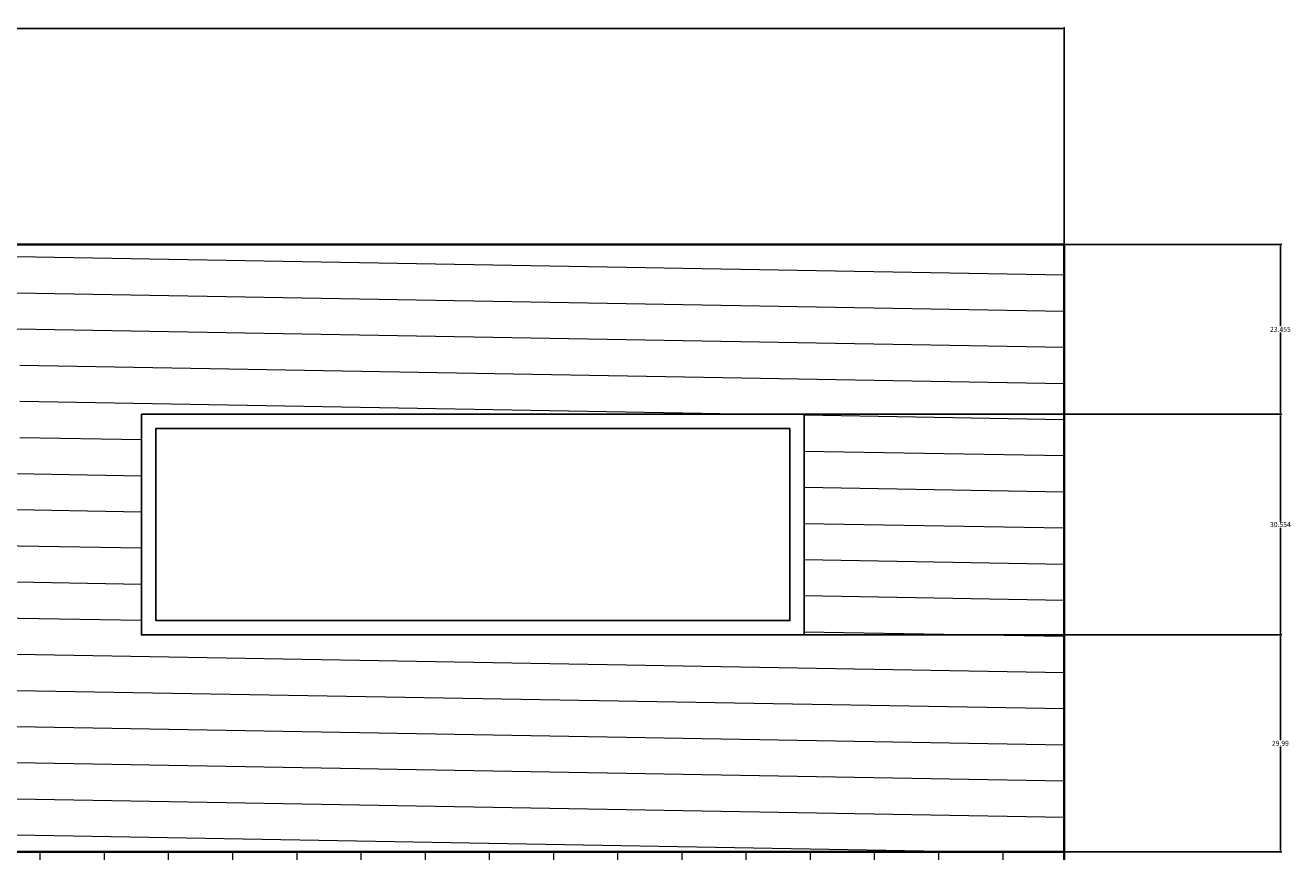
# Model space of a CAD drawing. Units: inches. Extents: x -145 to 510, y 5 to 386.
# Tile 25 of 25: x 335 to 510, y 272 to 386. Entities that reach past the tile are written whole.
import ezdxf

# ---------------------------------------------------------------- set-up
doc = ezdxf.new("R2010")
doc.units = ezdxf.units.IN
doc.header["$MEASUREMENT"] = 0
for name, color, linetype, lineweight in [('A-ANNO-DIMS', 2, 'Continuous', 18), ('A-ELEV', 7, 'Continuous', 35), ('A-ELEV-PATT', 8, 'Continuous', 13), ('A-GLAZ', 4, 'Continuous', 25)]:
    doc.layers.add(name, color=color, linetype=linetype, lineweight=lineweight)
doc.styles.get("Standard").update_dxf_attribs({"font": 'arial.ttf'})
doc.dimstyles.get("Standard").update_dxf_attribs({"dimtxt": 0.6875, "dimasz": 0.18, "dimexe": 0.18, "dimexo": 0.0625, "dimgap": 0.09, "dimtad": 0, "dimtih": 1, "dimtoh": 1, "dimdec": 4, "dimzin": 0, "dimdsep": 46, "dimlunit": 4, "dimtxsty": 'Standard', "dimcen": 0.09, "dimadec": 0, "dimazin": 0, "dimtfac": 1, "dimtdec": 4, "dimtofl": 0, "dimtmove": 0, "dimatfit": 3, "dimfxl": 1, "dimtolj": 1, "dimtzin": 0, "dimarcsym": 0})

# ---------------------------------------------------------------- blocks, each defined once
blk = doc.blocks.new('WIN-2200')
for points in [[(0, 30.55), (91.67, 30.55), (91.67, 0), (0, 0)], [(2, 28.55), (89.67, 28.55), (89.67, 2), (2, 2)]]:
    blk.add_lwpolyline(points, close=True)
blk = doc.blocks.new('*D14')
at = {"layer": 'A-ANNO-DIMS', "color": 0, "lineweight": -2, "transparency": 16777216}
for p, q in [((34.27, 341.23), (34.27, 385.97)), ((34.45, 385.79), (255.28, 385.79)), ((478.65, 385.79), (257.81, 385.79)), ((478.83, 355.95), (478.83, 385.97))]:
    blk.add_line(p, q, dxfattribs=at)
at = {"layer": 'A-ANNO-DIMS', "color": 0, "transparency": 16777216}
for points in [[(34.45, 385.82), (34.45, 385.76), (34.27, 385.79)], [(478.65, 385.82), (478.65, 385.76), (478.83, 385.79)]]:
    blk.add_solid(points, dxfattribs=at)
at = {"layer": 'Defpoints', "color": 0, "transparency": 16777216}
for p in [(478.83, 385.79), (478.83, 355.89), (34.27, 341.17)]:
    blk.add_point(p, dxfattribs=at)
at = {"layer": 'A-ANNO-DIMS', "color": 0, "transparency": 16777216, "insert": (256.55, 385.79), "char_height": 0.688, "attachment_point": 5}
blk.add_mtext('\\A1;444.6', dxfattribs=at)
blk = doc.blocks.new('*D19')
at = {"layer": 'A-ANNO-DIMS', "color": 0, "lineweight": -2, "transparency": 16777216}
for p, q in [((478.76, 355.89), (-144.05, 355.89)), ((-143.87, 355.71), (-143.87, 218.33)), ((-143.87, 80.07), (-143.87, 217.45)), ((-114.04, 79.89), (-144.05, 79.89))]:
    blk.add_line(p, q, dxfattribs=at)
at = {"layer": 'A-ANNO-DIMS', "color": 0, "transparency": 16777216}
for points in [[(-143.9, 355.71), (-143.84, 355.71), (-143.87, 355.89)], [(-143.9, 80.07), (-143.84, 80.07), (-143.87, 79.89)]]:
    blk.add_solid(points, dxfattribs=at)
at = {"layer": 'Defpoints', "color": 0, "transparency": 16777216}
for p in [(-143.87, 355.89), (478.83, 355.89), (-113.97, 79.89)]:
    blk.add_point(p, dxfattribs=at)
at = {"layer": 'A-ANNO-DIMS', "color": 0, "transparency": 16777216, "insert": (-143.87, 217.89), "char_height": 0.688, "attachment_point": 5}
blk.add_mtext('\\A1;276', dxfattribs=at)
blk = doc.blocks.new('*D37')
at = {"layer": 'A-ANNO-DIMS', "color": 0, "lineweight": -2, "transparency": 16777216}
for p, q in [((442.96, 301.88), (508.91, 301.88)), ((508.73, 301.7), (508.73, 287.33)), ((508.73, 272.07), (508.73, 286.45)), ((478.89, 271.89), (508.91, 271.89))]:
    blk.add_line(p, q, dxfattribs=at)
at = {"layer": 'A-ANNO-DIMS', "color": 0, "transparency": 16777216}
for points in [[(508.7, 301.7), (508.76, 301.7), (508.73, 301.88)], [(508.7, 272.07), (508.76, 272.07), (508.73, 271.89)]]:
    blk.add_solid(points, dxfattribs=at)
at = {"layer": 'Defpoints', "color": 0, "transparency": 16777216}
for p in [(442.9, 301.88), (508.73, 301.88), (478.83, 271.89)]:
    blk.add_point(p, dxfattribs=at)
at = {"layer": 'A-ANNO-DIMS', "color": 0, "transparency": 16777216, "insert": (508.73, 286.89), "char_height": 0.688, "attachment_point": 5}
blk.add_mtext('\\A1;29.99', dxfattribs=at)
blk = doc.blocks.new('*D38')
at = {"layer": 'A-ANNO-DIMS', "color": 0, "lineweight": -2, "transparency": 16777216}
for p, q in [((442.96, 332.44), (508.91, 332.44)), ((508.73, 332.26), (508.73, 317.6)), ((508.73, 302.06), (508.73, 316.72)), ((442.96, 301.88), (508.91, 301.88))]:
    blk.add_line(p, q, dxfattribs=at)
at = {"layer": 'A-ANNO-DIMS', "color": 0, "transparency": 16777216}
for points in [[(508.7, 332.26), (508.76, 332.26), (508.73, 332.44)], [(508.7, 302.06), (508.76, 302.06), (508.73, 301.88)]]:
    blk.add_solid(points, dxfattribs=at)
at = {"layer": 'Defpoints', "color": 0, "transparency": 16777216}
for p in [(442.9, 332.44), (508.73, 332.44), (442.9, 301.88)]:
    blk.add_point(p, dxfattribs=at)
at = {"layer": 'A-ANNO-DIMS', "color": 0, "transparency": 16777216, "insert": (508.73, 317.16), "char_height": 0.688, "attachment_point": 5}
blk.add_mtext('\\A1;30.554', dxfattribs=at)
blk = doc.blocks.new('*D39')
at = {"layer": 'A-ANNO-DIMS', "color": 0, "lineweight": -2, "transparency": 16777216}
for p, q in [((478.89, 355.89), (508.91, 355.89)), ((508.73, 355.71), (508.73, 344.6)), ((508.73, 332.62), (508.73, 343.72)), ((442.96, 332.44), (508.91, 332.44))]:
    blk.add_line(p, q, dxfattribs=at)
at = {"layer": 'A-ANNO-DIMS', "color": 0, "transparency": 16777216}
for points in [[(508.7, 355.71), (508.76, 355.71), (508.73, 355.89)], [(508.7, 332.62), (508.76, 332.62), (508.73, 332.44)]]:
    blk.add_solid(points, dxfattribs=at)
at = {"layer": 'Defpoints', "color": 0, "transparency": 16777216}
for p in [(478.83, 355.89), (508.73, 355.89), (442.9, 332.44)]:
    blk.add_point(p, dxfattribs=at)
at = {"layer": 'A-ANNO-DIMS', "color": 0, "transparency": 16777216, "insert": (508.73, 344.16), "char_height": 0.688, "attachment_point": 5}
blk.add_mtext('\\A1;23.455', dxfattribs=at)

msp = doc.modelspace()

# ---------------------------------------------------------------- hatches: boundary and pattern name
at = {"layer": 'A-ELEV-PATT'}
h = msp.add_hatch(dxfattribs=at)
h.set_pattern_fill('ANSI31', color=256, scale=40, angle=134)
h.paths.add_polyline_path([(478.8263, 355.8905), (309.4739, 355.8905), (309.4739, 341.168), (334.4402, 341.168), (334.4402, 327.6093), (309.4739, 327.6093), (309.4739, 271.8905), (478.8263, 271.8905)])
h.paths.add_polyline_path([(442.9009, 301.8821), (351.234, 301.8821), (351.234, 332.4358), (442.9009, 332.4358)], flags=16)
h.paths.add_polyline_path([(440.9009, 303.8821), (353.234, 303.8821), (353.234, 330.4358), (440.9009, 330.4358)], flags=0)
h = msp.add_hatch(dxfattribs=at)
h.set_pattern_fill('ANSI31', color=256, scale=71, angle=45)
h.paths.add_polyline_path([(478.8263, 271.8905), (309.4739, 271.8905), (309.4739, 259.8905), (309.4739, 235.8905), (317.2273, 235.8905), (474.4893, 235.8905), (478.8263, 235.8905)])

# ---------------------------------------------------------------- linework, layer by layer
at = {"layer": 'A-ELEV'}
for p, q in [((309.4739, 355.8905), (478.8263, 355.8905)), ((478.8263, 355.8905), (478.8263, 271.8905)), ((309.4739, 271.8905), (478.8263, 271.8905)), ((478.8263, 271.8905), (478.8263, 235.8905))]:
    msp.add_line(p, q, dxfattribs=at)

# ---------------------------------------------------------------- block references
at = {"layer": 'A-GLAZ'}
msp.add_blockref('WIN-2200', (351.234, 301.8824), dxfattribs=at)

# ---------------------------------------------------------------- dimensions: what is measured, and where the dimension line sits
at = {"layer": 'A-ANNO-DIMS'}
dim = msp.add_linear_dim(base=(478.8263, 385.7905), p1=(34.2706, 341.168), p2=(478.8263, 355.8905), dimstyle='Standard', override={"dimdec": 1, "dimlfac": 1, "dimrnd": 0, "dimzin": 0, "dimdsep": 46, "dimlunit": 2}, dxfattribs=at)
dim.commit()
dim.dimension.update_dxf_attribs({"geometry": '*D14', "text_midpoint": (256.5484, 385.7905)})
for base, p1, p2, override, picture, middle in [((-143.8737, 355.8905), (-113.9737, 79.8905), (478.8263, 355.8905), {"dimdec": 0, "dimlfac": 1, "dimrnd": 0, "dimzin": 0, "dimdsep": 46, "dimlunit": 2}, '*D19', (-143.8737, 217.8905)), ((508.7263, 355.8905), (442.9009, 332.4358), (478.8263, 355.8905), {"dimdec": 3, "dimlfac": 1, "dimrnd": 0, "dimzin": 0, "dimdsep": 46, "dimlunit": 2}, '*D39', (508.7263, 344.1632)), ((508.7263, 332.4358), (442.9009, 301.8821), (442.9009, 332.4358), {"dimdec": 3, "dimlfac": 1, "dimrnd": 0, "dimzin": 0, "dimdsep": 46, "dimlunit": 2}, '*D38', (508.7263, 317.159)), ((508.7263, 301.8821), (478.8263, 271.8905), (442.9009, 301.8821), {"dimdec": 2, "dimlfac": 1, "dimrnd": 0, "dimzin": 0, "dimdsep": 46, "dimlunit": 2}, '*D37', (508.7263, 286.8863))]:
    dim = msp.add_linear_dim(base=base, p1=p1, p2=p2, angle=90, dimstyle='Standard', override=override, dxfattribs=at)
    dim.commit()
    dim.dimension.update_dxf_attribs({"geometry": picture, "text_midpoint": middle})

doc.saveas('drawing.dxf')
